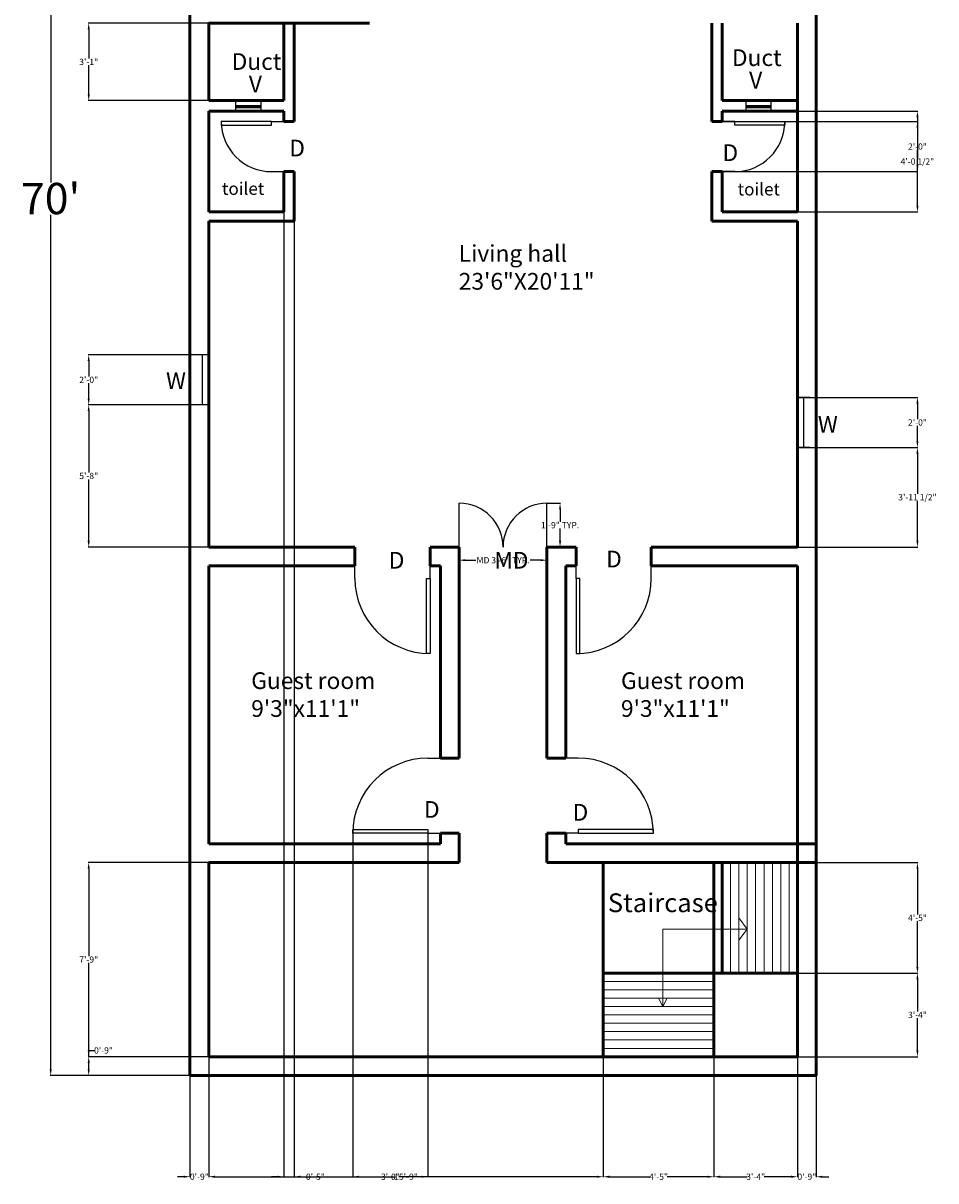
# Model space of a CAD drawing. Units: inches. Extents: x -250 to 2650, y 180 to 1183.
# Tile 7 of 10: x 1594 to 2031, y 180 to 734. Entities that reach past the tile are written whole.
import ezdxf

# ---------------------------------------------------------------- set-up
doc = ezdxf.new("R2010")
doc.units = ezdxf.units.IN
doc.header["$MEASUREMENT"] = 0
for name, color, linetype, lineweight in [('A-ANNO-DIMS', 2, 'Continuous', 18), ('A-ANNO-TEXT', 7, 'Continuous', 18), ('A-AREA-IDEN', 3, 'Continuous', 18), ('A-DOOR', 4, 'Continuous', 25), ('A-FLOR-STRS', 8, 'Continuous', 18), ('A-GLAZ', 3, 'Continuous', 25), ('A-WALL', 7, 'Continuous', 50)]:
    doc.layers.add(name, color=color, linetype=linetype, lineweight=lineweight)
doc.styles.get("Standard").update_dxf_attribs({"font": 'arial.ttf'})
doc.dimstyles.get("Standard").update_dxf_attribs({"dimtxt": 3, "dimasz": 3, "dimexe": 0.18, "dimexo": 0.0625, "dimgap": 0.09, "dimtad": 0, "dimtih": 1, "dimtoh": 1, "dimdec": 0, "dimzin": 0, "dimdsep": 46, "dimlunit": 3, "dimtxsty": 'Standard', "dimcen": 0.09, "dimadec": 0, "dimazin": 0, "dimtfac": 1, "dimtdec": 0, "dimtofl": 0, "dimtmove": 0, "dimatfit": 3, "dimfxl": 1, "dimtolj": 1, "dimtzin": 0, "dimarcsym": 0})

# ---------------------------------------------------------------- blocks, each defined once
blk = doc.blocks.new('*D37')
at = {"layer": 'A-ANNO-DIMS', "color": 0, "lineweight": -2, "transparency": 16777216}
for p, q in [((1673.43, 1070.02), (1606.61, 1070.02)), ((1606.79, 1067.02), (1606.79, 657.77)), ((1606.79, 233.02), (1606.79, 642.28)), ((1673.43, 230.02), (1606.61, 230.02))]:
    blk.add_line(p, q, dxfattribs=at)
at = {"layer": 'A-ANNO-DIMS', "color": 0, "transparency": 16777216}
for points in [[(1606.29, 1067.02), (1607.29, 1067.02), (1606.79, 1070.02)], [(1606.29, 233.02), (1607.29, 233.02), (1606.79, 230.02)]]:
    blk.add_solid(points, dxfattribs=at)
at = {"layer": 'Defpoints', "color": 0, "transparency": 16777216}
for p in [(1673.49, 1070.02), (1606.79, 230.02), (1673.49, 230.02)]:
    blk.add_point(p, dxfattribs=at)
at = {"layer": 'A-ANNO-DIMS', "color": 0, "transparency": 16777216, "insert": (1606.79, 650.02), "char_height": 3, "attachment_point": 5}
blk.add_mtext("\\A1;{\\H5x;70'}", dxfattribs=at)
blk = doc.blocks.new('*U27')
for p, q in [((0, 0), (0, -6)), ((24, 0), (24, -6))]:
    blk.add_line(p, q)
blk.add_lwpolyline([(0, 0), (0, 24), (1.75, 24), (1.75, 0)], close=True)
blk.add_arc((0, 0), 24, 0, 90)
blk = doc.blocks.new('*U28')
for p, q in [((0, 0), (0, 6)), ((24, 0), (24, 6))]:
    blk.add_line(p, q)
blk.add_lwpolyline([(0, 0), (0, -24), (1.75, -24), (1.75, 0)], close=True)
blk.add_arc((0, 0), 24, 270, 0)
blk = doc.blocks.new('*U29')
for p, q in [((0, 5), (0, 0)), ((0, 2.5), (12, 2.5)), ((12, 5), (12, 0))]:
    blk.add_line(p, q)
blk = doc.blocks.new('*U30')
for p, q in [((-36, 0), (-36, -6)), ((0, 0), (0, -6))]:
    blk.add_line(p, q)
blk.add_lwpolyline([(0, 0), (0, 36), (-1.75, 36), (-1.75, 0)], close=True)
blk.add_arc((0, 0), 36, 90, 180)
blk = doc.blocks.new('*U31')
for p, q in [((-36, 0), (-36, 6)), ((0, 0), (0, 6))]:
    blk.add_line(p, q)
blk.add_lwpolyline([(0, 0), (0, -36), (-1.75, -36), (-1.75, 0)], close=True)
blk.add_arc((0, 0), 36, 180, 270)
blk = doc.blocks.new('*U32')
for p, q in [((0, 0), (0, -6)), ((36, 0), (36, -6))]:
    blk.add_line(p, q)
blk.add_lwpolyline([(0, 0), (0, 36), (1.75, 36), (1.75, 0)], close=True)
blk.add_arc((0, 0), 36, 0, 90)
blk = doc.blocks.new('*U33')
for p, q in [((-36, 0), (-36, -6)), ((0, 0), (0, -6))]:
    blk.add_line(p, q)
blk.add_lwpolyline([(0, 0), (0, 36), (-1.75, 36), (-1.75, 0)], close=True)
blk.add_arc((0, 0), 36, 90, 180)
blk = doc.blocks.new('*U23')
for p, q in [((-24, 6), (-24, 0)), ((0, 6), (0, 0)), ((0, 3), (-24, 3))]:
    blk.add_line(p, q)
blk = doc.blocks.new('*U24')
for p, q in [((-24, 6), (-24, 0)), ((0, 6), (0, 0)), ((0, 3), (-24, 3))]:
    blk.add_line(p, q)
blk = doc.blocks.new('DOOR-DOUBLE-MAIN')
for p, q in [((505.08, 483.11), (505.08, 504.11)), ((505.08, 483.11), (505.08, 504.11)), ((547.08, 483.11), (547.08, 504.11))]:
    blk.add_line(p, q)
for centre, start, end in [((505.08, 483.11), 0, 90), ((505.08, 483.11), 0, 90), ((547.08, 483.11), 90, 180)]:
    blk.add_arc(centre, 21, start, end)
blk = doc.blocks.new('*D52')
at = {"layer": 'A-ANNO-DIMS', "color": 0, "lineweight": -2, "transparency": 16777216}
for p, q in [((1802.49, 483.05), (1802.49, 476.63)), ((1844.49, 483.05), (1844.49, 476.63)), ((1805.49, 476.81), (1810.49, 476.81)), ((1841.49, 476.81), (1836.5, 476.81))]:
    blk.add_line(p, q, dxfattribs=at)
at = {"layer": 'A-ANNO-DIMS', "color": 0, "transparency": 16777216}
for points in [[(1805.49, 477.31), (1805.49, 476.31), (1802.49, 476.81)], [(1841.49, 477.31), (1841.49, 476.31), (1844.49, 476.81)]]:
    blk.add_solid(points, dxfattribs=at)
at = {"layer": 'Defpoints', "color": 0, "transparency": 16777216}
for p in [(1802.49, 483.11), (1844.49, 483.11), (1844.49, 476.81)]:
    blk.add_point(p, dxfattribs=at)
at = {"layer": 'A-ANNO-DIMS', "color": 0, "transparency": 16777216, "insert": (1823.49, 476.81), "char_height": 3, "attachment_point": 5}
blk.add_mtext('\\A1;MD 3\'-6" TYP.', dxfattribs=at)
blk = doc.blocks.new('*D53')
at = {"layer": 'A-ANNO-DIMS', "color": 0, "lineweight": -2, "transparency": 16777216}
for p, q in [((1844.55, 504.11), (1850.97, 504.11)), ((1850.79, 501.11), (1850.79, 495.23)), ((1850.79, 486.11), (1850.79, 491.99)), ((1844.55, 483.11), (1850.97, 483.11))]:
    blk.add_line(p, q, dxfattribs=at)
at = {"layer": 'A-ANNO-DIMS', "color": 0, "transparency": 16777216}
for points in [[(1850.29, 501.11), (1851.29, 501.11), (1850.79, 504.11)], [(1850.29, 486.11), (1851.29, 486.11), (1850.79, 483.11)]]:
    blk.add_solid(points, dxfattribs=at)
at = {"layer": 'Defpoints', "color": 0, "transparency": 16777216}
for p in [(1844.49, 504.11), (1850.79, 504.11), (1844.49, 483.11)]:
    blk.add_point(p, dxfattribs=at)
at = {"layer": 'A-ANNO-DIMS', "color": 0, "transparency": 16777216, "insert": (1850.79, 493.61), "char_height": 3, "attachment_point": 5}
blk.add_mtext('\\A1;1\'-9" TYP.', dxfattribs=at)
blk = doc.blocks.new('*D134')
at = {"layer": 'A-ANNO-DIMS', "color": 0, "lineweight": -2, "transparency": 16777216}
for p, q in [((1964.49229, 238.962048), (1964.49229, 181.344548)), ((1973.49229, 229.962048), (1973.49229, 181.344548)), ((1961.49229, 181.524548), (1958.49229, 181.524548)), ((1976.49229, 181.524548), (1979.49229, 181.524548))]:
    blk.add_line(p, q, dxfattribs=at)
at = {"layer": 'A-ANNO-DIMS', "color": 0, "transparency": 16777216}
for points in [[(1961.49229, 182.024548), (1961.49229, 181.024548), (1964.49229, 181.524548)], [(1976.49229, 182.024548), (1976.49229, 181.024548), (1973.49229, 181.524548)]]:
    blk.add_solid(points, dxfattribs=at)
at = {"layer": 'Defpoints', "color": 0, "transparency": 16777216}
for p in [(1964.49229, 239.024548), (1973.49229, 230.024548), (1973.49229, 181.524548)]:
    blk.add_point(p, dxfattribs=at)
at = {"layer": 'A-ANNO-DIMS', "color": 0, "transparency": 16777216, "insert": (1968.99229, 181.524548), "char_height": 3, "attachment_point": 5}
blk.add_mtext('\\A1;0\'-9"', dxfattribs=at)
blk = doc.blocks.new('*D135')
at = {"layer": 'A-ANNO-DIMS', "color": 0, "lineweight": -2, "transparency": 16777216}
for p, q in [((1682.49229, 238.962048), (1682.49229, 181.344548)), ((1673.49229, 229.962048), (1673.49229, 181.344548)), ((1670.49229, 181.524548), (1667.49229, 181.524548)), ((1685.49229, 181.524548), (1688.49229, 181.524548))]:
    blk.add_line(p, q, dxfattribs=at)
at = {"layer": 'A-ANNO-DIMS', "color": 0, "transparency": 16777216}
for points in [[(1670.49229, 182.024548), (1670.49229, 181.024548), (1673.49229, 181.524548)], [(1685.49229, 182.024548), (1685.49229, 181.024548), (1682.49229, 181.524548)]]:
    blk.add_solid(points, dxfattribs=at)
at = {"layer": 'Defpoints', "color": 0, "transparency": 16777216}
for p in [(1682.49229, 239.024548), (1673.49229, 230.024548), (1682.49229, 181.524548)]:
    blk.add_point(p, dxfattribs=at)
at = {"layer": 'A-ANNO-DIMS', "color": 0, "transparency": 16777216, "insert": (1677.99229, 181.524548), "char_height": 3, "attachment_point": 5}
blk.add_mtext('\\A1;0\'-9"', dxfattribs=at)
blk = doc.blocks.new('*D136')
at = {"layer": 'A-ANNO-DIMS', "color": 0, "lineweight": -2, "transparency": 16777216}
for p, q in [((1682.49, 238.96), (1682.49, 181.34)), ((1871.49, 238.96), (1871.49, 181.34)), ((1685.49, 181.52), (1771.89, 181.52)), ((1868.49, 181.52), (1782.09, 181.52))]:
    blk.add_line(p, q, dxfattribs=at)
at = {"layer": 'A-ANNO-DIMS', "color": 0, "transparency": 16777216}
for points in [[(1685.49, 182.02), (1685.49, 181.02), (1682.49, 181.52)], [(1868.49, 182.02), (1868.49, 181.02), (1871.49, 181.52)]]:
    blk.add_solid(points, dxfattribs=at)
at = {"layer": 'Defpoints', "color": 0, "transparency": 16777216}
for p in [(1682.49, 239.02), (1871.49, 239.02), (1871.49, 181.52)]:
    blk.add_point(p, dxfattribs=at)
at = {"layer": 'A-ANNO-DIMS', "color": 0, "transparency": 16777216, "insert": (1776.99, 181.52), "char_height": 3, "attachment_point": 5}
blk.add_mtext('\\A1;15\'-9"', dxfattribs=at)
blk = doc.blocks.new('*D137')
at = {"layer": 'A-ANNO-DIMS', "color": 0, "lineweight": -2, "transparency": 16777216}
for p, q in [((1871.49, 238.96), (1871.49, 181.34)), ((1924.49, 238.96), (1924.49, 181.34)), ((1874.49, 181.52), (1893.85, 181.52)), ((1921.49, 181.52), (1902.13, 181.52))]:
    blk.add_line(p, q, dxfattribs=at)
at = {"layer": 'A-ANNO-DIMS', "color": 0, "transparency": 16777216}
for points in [[(1874.49, 182.02), (1874.49, 181.02), (1871.49, 181.52)], [(1921.49, 182.02), (1921.49, 181.02), (1924.49, 181.52)]]:
    blk.add_solid(points, dxfattribs=at)
at = {"layer": 'Defpoints', "color": 0, "transparency": 16777216}
for p in [(1871.49, 239.02), (1924.49, 239.02), (1924.49, 181.52)]:
    blk.add_point(p, dxfattribs=at)
at = {"layer": 'A-ANNO-DIMS', "color": 0, "transparency": 16777216, "insert": (1897.99, 181.52), "char_height": 3, "attachment_point": 5}
blk.add_mtext('\\A1;4\'-5"', dxfattribs=at)
blk = doc.blocks.new('*D138')
at = {"layer": 'A-ANNO-DIMS', "color": 0, "lineweight": -2, "transparency": 16777216}
for p, q in [((1924.49, 238.96), (1924.49, 181.34)), ((1964.49, 238.96), (1964.49, 181.34)), ((1927.49, 181.52), (1940.42, 181.52)), ((1961.49, 181.52), (1948.57, 181.52))]:
    blk.add_line(p, q, dxfattribs=at)
at = {"layer": 'A-ANNO-DIMS', "color": 0, "transparency": 16777216}
for points in [[(1927.49, 182.02), (1927.49, 181.02), (1924.49, 181.52)], [(1961.49, 182.02), (1961.49, 181.02), (1964.49, 181.52)]]:
    blk.add_solid(points, dxfattribs=at)
at = {"layer": 'Defpoints', "color": 0, "transparency": 16777216}
for p in [(1924.49, 239.02), (1964.49, 239.02), (1964.49, 181.52)]:
    blk.add_point(p, dxfattribs=at)
at = {"layer": 'A-ANNO-DIMS', "color": 0, "transparency": 16777216, "insert": (1944.49, 181.52), "char_height": 3, "attachment_point": 5}
blk.add_mtext('\\A1;3\'-4"', dxfattribs=at)
blk = doc.blocks.new('*D139')
at = {"layer": 'A-ANNO-DIMS', "color": 0, "lineweight": -2, "transparency": 16777216}
for p, q in [((1964.55, 279.02), (2022.17, 279.02)), ((2021.99, 276.02), (2021.99, 260.65)), ((2021.99, 242.02), (2021.99, 257.4)), ((1964.55, 239.02), (2022.17, 239.02))]:
    blk.add_line(p, q, dxfattribs=at)
at = {"layer": 'A-ANNO-DIMS', "color": 0, "transparency": 16777216}
for points in [[(2021.49, 276.02), (2022.49, 276.02), (2021.99, 279.02)], [(2021.49, 242.02), (2022.49, 242.02), (2021.99, 239.02)]]:
    blk.add_solid(points, dxfattribs=at)
at = {"layer": 'Defpoints', "color": 0, "transparency": 16777216}
for p in [(1964.49, 279.02), (2021.99, 279.02), (1964.49, 239.02)]:
    blk.add_point(p, dxfattribs=at)
at = {"layer": 'A-ANNO-DIMS', "color": 0, "transparency": 16777216, "insert": (2021.99, 259.02), "char_height": 3, "attachment_point": 5}
blk.add_mtext('\\A1;3\'-4"', dxfattribs=at)
blk = doc.blocks.new('*D140')
at = {"layer": 'A-ANNO-DIMS', "color": 0, "lineweight": -2, "transparency": 16777216}
for p, q in [((1960.55, 332.02), (2022.17, 332.02)), ((2021.99, 329.02), (2021.99, 307.14)), ((2021.99, 282.02), (2021.99, 303.91)), ((1964.55, 279.02), (2022.17, 279.02))]:
    blk.add_line(p, q, dxfattribs=at)
at = {"layer": 'A-ANNO-DIMS', "color": 0, "transparency": 16777216}
for points in [[(2021.49, 329.02), (2022.49, 329.02), (2021.99, 332.02)], [(2021.49, 282.02), (2022.49, 282.02), (2021.99, 279.02)]]:
    blk.add_solid(points, dxfattribs=at)
at = {"layer": 'Defpoints', "color": 0, "transparency": 16777216}
for p in [(1960.49, 332.02), (2021.99, 332.02), (1964.49, 279.02)]:
    blk.add_point(p, dxfattribs=at)
at = {"layer": 'A-ANNO-DIMS', "color": 0, "transparency": 16777216, "insert": (2021.99, 305.52), "char_height": 3, "attachment_point": 5}
blk.add_mtext('\\A1;4\'-5"', dxfattribs=at)
blk = doc.blocks.new('*D141')
at = {"layer": 'A-ANNO-DIMS', "color": 0, "lineweight": -2, "transparency": 16777216}
for p, q in [((1682.43, 239.02), (1624.81, 239.02)), ((1624.99, 239.02), (1624.99, 242.02)), ((1624.99, 242.02), (1627.99, 242.02)), ((1624.99, 233.02), (1624.99, 236.02)), ((1673.43, 230.02), (1624.81, 230.02))]:
    blk.add_line(p, q, dxfattribs=at)
at = {"layer": 'A-ANNO-DIMS', "color": 0, "transparency": 16777216}
for points in [[(1624.49, 236.02), (1625.49, 236.02), (1624.99, 239.02)], [(1624.49, 233.02), (1625.49, 233.02), (1624.99, 230.02)]]:
    blk.add_solid(points, dxfattribs=at)
at = {"layer": 'Defpoints', "color": 0, "transparency": 16777216}
for p in [(1624.99, 239.02), (1682.49, 239.02), (1673.49, 230.02)]:
    blk.add_point(p, dxfattribs=at)
at = {"layer": 'A-ANNO-DIMS', "color": 0, "transparency": 16777216, "insert": (1632.07, 242.02), "char_height": 3, "attachment_point": 5}
blk.add_mtext('\\A1;0\'-9"', dxfattribs=at)
blk = doc.blocks.new('*D142')
at = {"layer": 'A-ANNO-DIMS', "color": 0, "lineweight": -2, "transparency": 16777216}
for p, q in [((1682.43, 332.02), (1624.81, 332.02)), ((1624.99, 329.02), (1624.99, 287.15)), ((1624.99, 242.02), (1624.99, 283.9)), ((1682.43, 239.02), (1624.81, 239.02))]:
    blk.add_line(p, q, dxfattribs=at)
at = {"layer": 'A-ANNO-DIMS', "color": 0, "transparency": 16777216}
for points in [[(1624.49, 329.02), (1625.49, 329.02), (1624.99, 332.02)], [(1624.49, 242.02), (1625.49, 242.02), (1624.99, 239.02)]]:
    blk.add_solid(points, dxfattribs=at)
at = {"layer": 'Defpoints', "color": 0, "transparency": 16777216}
for p in [(1624.99, 332.02), (1682.49, 332.02), (1682.49, 239.02)]:
    blk.add_point(p, dxfattribs=at)
at = {"layer": 'A-ANNO-DIMS', "color": 0, "transparency": 16777216, "insert": (1624.99, 285.52), "char_height": 3, "attachment_point": 5}
blk.add_mtext('\\A1;7\'-9"', dxfattribs=at)
blk = doc.blocks.new('*D144')
at = {"layer": 'A-ANNO-DIMS', "color": 0, "lineweight": -2, "transparency": 16777216}
for p, q in [((1718.49, 643.56), (1718.49, 181.34)), ((1723.49, 639.05), (1723.49, 181.34)), ((1715.49, 181.52), (1712.49, 181.52)), ((1726.49, 181.52), (1729.49, 181.52))]:
    blk.add_line(p, q, dxfattribs=at)
at = {"layer": 'A-ANNO-DIMS', "color": 0, "transparency": 16777216}
for points in [[(1715.49, 182.02), (1715.49, 181.02), (1718.49, 181.52)], [(1726.49, 182.02), (1726.49, 181.02), (1723.49, 181.52)]]:
    blk.add_solid(points, dxfattribs=at)
at = {"layer": 'Defpoints', "color": 0, "transparency": 16777216}
for p in [(1718.49, 643.62), (1723.49, 639.11), (1723.49, 181.52)]:
    blk.add_point(p, dxfattribs=at)
at = {"layer": 'A-ANNO-DIMS', "color": 0, "transparency": 16777216, "insert": (1733.57, 181.52), "char_height": 3, "attachment_point": 5}
blk.add_mtext('\\A1;0\'-5"', dxfattribs=at)
blk = doc.blocks.new('*D145')
at = {"layer": 'A-ANNO-DIMS', "color": 0, "lineweight": -2, "transparency": 16777216}
for p, q in [((1682.43, 734.02), (1624.81, 734.02)), ((1624.99, 731.02), (1624.99, 717.09)), ((1624.99, 699.91), (1624.99, 713.84)), ((1682.43, 696.91), (1624.81, 696.91))]:
    blk.add_line(p, q, dxfattribs=at)
at = {"layer": 'A-ANNO-DIMS', "color": 0, "transparency": 16777216}
for points in [[(1624.49, 731.02), (1625.49, 731.02), (1624.99, 734.02)], [(1624.49, 699.91), (1625.49, 699.91), (1624.99, 696.91)]]:
    blk.add_solid(points, dxfattribs=at)
at = {"layer": 'Defpoints', "color": 0, "transparency": 16777216}
for p in [(1624.99, 734.02), (1682.49, 734.02), (1682.49, 696.91)]:
    blk.add_point(p, dxfattribs=at)
at = {"layer": 'A-ANNO-DIMS', "color": 0, "transparency": 16777216, "insert": (1624.99, 715.47), "char_height": 3, "attachment_point": 5}
blk.add_mtext('\\A1;3\'-1"', dxfattribs=at)
blk = doc.blocks.new('*D146')
at = {"layer": 'A-ANNO-DIMS', "color": 0, "lineweight": -2, "transparency": 16777216}
for p, q in [((1964.55, 691.91), (2022.17, 691.91)), ((2021.99, 688.91), (2021.99, 669.41)), ((2021.99, 646.62), (2021.99, 666.12)), ((1964.55, 643.62), (2022.17, 643.62))]:
    blk.add_line(p, q, dxfattribs=at)
at = {"layer": 'A-ANNO-DIMS', "color": 0, "transparency": 16777216}
for points in [[(2021.49, 688.91), (2022.49, 688.91), (2021.99, 691.91)], [(2021.49, 646.62), (2022.49, 646.62), (2021.99, 643.62)]]:
    blk.add_solid(points, dxfattribs=at)
at = {"layer": 'Defpoints', "color": 0, "transparency": 16777216}
for p in [(1964.49, 691.91), (2021.99, 691.91), (1964.49, 643.62)]:
    blk.add_point(p, dxfattribs=at)
at = {"layer": 'A-ANNO-DIMS', "color": 0, "transparency": 16777216, "insert": (2021.99, 667.77), "char_height": 3, "attachment_point": 5}
blk.add_mtext('\\A1;4\'-0 1/2"', dxfattribs=at)
blk = doc.blocks.new('*D147')
at = {"layer": 'A-ANNO-DIMS', "color": 0, "lineweight": -2, "transparency": 16777216}
for p, q in [((1964.55, 530.79), (2022.17, 530.79)), ((2021.99, 527.79), (2021.99, 508.59)), ((2021.99, 486.11), (2021.99, 505.31)), ((1964.55, 483.11), (2022.17, 483.11))]:
    blk.add_line(p, q, dxfattribs=at)
at = {"layer": 'A-ANNO-DIMS', "color": 0, "transparency": 16777216}
for points in [[(2021.49, 527.79), (2022.49, 527.79), (2021.99, 530.79)], [(2021.49, 486.11), (2022.49, 486.11), (2021.99, 483.11)]]:
    blk.add_solid(points, dxfattribs=at)
at = {"layer": 'Defpoints', "color": 0, "transparency": 16777216}
for p in [(1964.49, 530.79), (2021.99, 530.79), (1964.49, 483.11)]:
    blk.add_point(p, dxfattribs=at)
at = {"layer": 'A-ANNO-DIMS', "color": 0, "transparency": 16777216, "insert": (2021.99, 506.95), "char_height": 3, "attachment_point": 5}
blk.add_mtext('\\A1;3\'-11 1/2"', dxfattribs=at)
blk = doc.blocks.new('*D148')
at = {"layer": 'A-ANNO-DIMS', "color": 0, "lineweight": -2, "transparency": 16777216}
for p, q in [((1964.55, 554.79), (2022.17, 554.79)), ((2021.99, 551.79), (2021.99, 544.41)), ((2021.99, 533.79), (2021.99, 541.16)), ((1964.55, 530.79), (2022.17, 530.79))]:
    blk.add_line(p, q, dxfattribs=at)
at = {"layer": 'A-ANNO-DIMS', "color": 0, "transparency": 16777216}
for points in [[(2021.49, 551.79), (2022.49, 551.79), (2021.99, 554.79)], [(2021.49, 533.79), (2022.49, 533.79), (2021.99, 530.79)]]:
    blk.add_solid(points, dxfattribs=at)
at = {"layer": 'Defpoints', "color": 0, "transparency": 16777216}
for p in [(1964.49, 554.79), (2021.99, 554.79), (1964.49, 530.79)]:
    blk.add_point(p, dxfattribs=at)
at = {"layer": 'A-ANNO-DIMS', "color": 0, "transparency": 16777216, "insert": (2021.99, 542.79), "char_height": 3, "attachment_point": 5}
blk.add_mtext('\\A1;2\'-0"', dxfattribs=at)
blk = doc.blocks.new('*D149')
at = {"layer": 'A-ANNO-DIMS', "color": 0, "lineweight": -2, "transparency": 16777216}
for p, q in [((1682.43, 551.2), (1624.81, 551.2)), ((1624.99, 548.2), (1624.99, 518.78)), ((1624.99, 486.11), (1624.99, 515.53)), ((1682.43, 483.11), (1624.81, 483.11))]:
    blk.add_line(p, q, dxfattribs=at)
at = {"layer": 'A-ANNO-DIMS', "color": 0, "transparency": 16777216}
for points in [[(1624.49, 548.2), (1625.49, 548.2), (1624.99, 551.2)], [(1624.49, 486.11), (1625.49, 486.11), (1624.99, 483.11)]]:
    blk.add_solid(points, dxfattribs=at)
at = {"layer": 'Defpoints', "color": 0, "transparency": 16777216}
for p in [(1624.99, 551.2), (1682.49, 551.2), (1682.49, 483.11)]:
    blk.add_point(p, dxfattribs=at)
at = {"layer": 'A-ANNO-DIMS', "color": 0, "transparency": 16777216, "insert": (1624.99, 517.16), "char_height": 3, "attachment_point": 5}
blk.add_mtext('\\A1;5\'-8"', dxfattribs=at)
blk = doc.blocks.new('*D150')
at = {"layer": 'A-ANNO-DIMS', "color": 0, "lineweight": -2, "transparency": 16777216}
for p, q in [((1682.43, 575.2), (1624.81, 575.2)), ((1624.99, 572.2), (1624.99, 564.82)), ((1624.99, 554.2), (1624.99, 561.58)), ((1682.43, 551.2), (1624.81, 551.2))]:
    blk.add_line(p, q, dxfattribs=at)
at = {"layer": 'A-ANNO-DIMS', "color": 0, "transparency": 16777216}
for points in [[(1624.49, 572.2), (1625.49, 572.2), (1624.99, 575.2)], [(1624.49, 554.2), (1625.49, 554.2), (1624.99, 551.2)]]:
    blk.add_solid(points, dxfattribs=at)
at = {"layer": 'Defpoints', "color": 0, "transparency": 16777216}
for p in [(1624.99, 575.2), (1682.49, 575.2), (1682.49, 551.2)]:
    blk.add_point(p, dxfattribs=at)
at = {"layer": 'A-ANNO-DIMS', "color": 0, "transparency": 16777216, "insert": (1624.99, 563.2), "char_height": 3, "attachment_point": 5}
blk.add_mtext('\\A1;2\'-0"', dxfattribs=at)
blk = doc.blocks.new('*D151')
at = {"layer": 'A-ANNO-DIMS', "color": 0, "lineweight": -2, "transparency": 16777216}
for p, q in [((1751.49, 345.96), (1751.49, 181.34)), ((1787.49, 345.96), (1787.49, 181.34)), ((1754.49, 181.52), (1765.42, 181.52)), ((1784.49, 181.52), (1773.57, 181.52))]:
    blk.add_line(p, q, dxfattribs=at)
at = {"layer": 'A-ANNO-DIMS', "color": 0, "transparency": 16777216}
for points in [[(1754.49, 182.02), (1754.49, 181.02), (1751.49, 181.52)], [(1784.49, 182.02), (1784.49, 181.02), (1787.49, 181.52)]]:
    blk.add_solid(points, dxfattribs=at)
at = {"layer": 'Defpoints', "color": 0, "transparency": 16777216}
for p in [(1751.49, 346.02), (1787.49, 346.02), (1787.49, 181.52)]:
    blk.add_point(p, dxfattribs=at)
at = {"layer": 'A-ANNO-DIMS', "color": 0, "transparency": 16777216, "insert": (1769.49, 181.52), "char_height": 3, "attachment_point": 5}
blk.add_mtext('\\A1;3\'-0"', dxfattribs=at)
blk = doc.blocks.new('*D152')
at = {"layer": 'A-ANNO-DIMS', "color": 0, "lineweight": -2, "transparency": 16777216}
for p, q in [((1923.55, 686.91), (2022.17, 686.91)), ((2021.99, 683.91), (2021.99, 676.53)), ((2021.99, 665.91), (2021.99, 673.29)), ((1923.55, 662.91), (2022.17, 662.91))]:
    blk.add_line(p, q, dxfattribs=at)
at = {"layer": 'A-ANNO-DIMS', "color": 0, "transparency": 16777216}
for points in [[(2021.49, 683.91), (2022.49, 683.91), (2021.99, 686.91)], [(2021.49, 665.91), (2022.49, 665.91), (2021.99, 662.91)]]:
    blk.add_solid(points, dxfattribs=at)
at = {"layer": 'Defpoints', "color": 0, "transparency": 16777216}
for p in [(1923.49, 686.91), (2021.99, 686.91), (1923.49, 662.91)]:
    blk.add_point(p, dxfattribs=at)
at = {"layer": 'A-ANNO-DIMS', "color": 0, "transparency": 16777216, "insert": (2021.99, 674.91), "char_height": 3, "attachment_point": 5}
blk.add_mtext('\\A1;2\'-0"', dxfattribs=at)

msp = doc.modelspace()

# ---------------------------------------------------------------- linework, layer by layer
at = {"layer": 'A-FLOR-STRS'}
for p, q in [((1932.49, 279.02), (1932.49, 332.02)), ((1936.49, 279.02), (1936.49, 332.02)), ((1940.49, 279.02), (1940.49, 332.02)), ((1944.49, 279.02), (1944.49, 332.02)), ((1948.49, 279.02), (1948.49, 332.02)), ((1952.49, 279.02), (1952.49, 332.02)), ((1956.49, 279.02), (1956.49, 332.02)), ((1960.49, 279.02), (1960.49, 332.02)), ((1940.49, 300.14), (1936.49, 305.52)), ((1900, 300.14), (1900, 263.02)), ((1900, 300.14), (1940.49, 300.14)), ((1940.49, 300.14), (1936.49, 294.75)), ((1871.49, 275.02), (1924.49, 275.02)), ((1871.49, 271.02), (1924.49, 271.02)), ((1871.49, 267.02), (1924.49, 267.02)), ((1900, 263.02), (1897.99, 267.02)), ((1900, 263.02), (1902.02, 267.02)), ((1871.49, 263.02), (1924.49, 263.02)), ((1871.49, 259.02), (1924.49, 259.02)), ((1871.49, 255.02), (1924.49, 255.02)), ((1871.49, 251.02), (1924.49, 251.02)), ((1871.49, 247.02), (1924.49, 247.02)), ((1871.49, 243.02), (1924.49, 243.02))]:
    msp.add_line(p, q, dxfattribs=at)
at = {"layer": 'A-WALL'}
for p, q in [((1673.49, 1070.02), (1673.49, 230.02)), ((1973.49, 230.02), (1973.49, 1070.02)), ((1759.49, 734.02), (1682.49, 734.02)), ((1682.49, 734.02), (1682.49, 696.91)), ((1718.49, 696.91), (1718.49, 734.02)), ((1723.49, 686.91), (1723.49, 734.02)), ((1923.49, 686.91), (1923.49, 734.02)), ((1923.49, 686.91), (1923.49, 734.02)), ((1928.49, 696.91), (1928.49, 734.02)), ((1964.49, 643.62), (1964.49, 734.02)), ((1964.49, 696.91), (1964.49, 734.02)), ((1964.49, 716.02), (1964.49, 734.02)), ((1718.49, 696.91), (1682.49, 696.91)), ((1707.55, 693.93), (1695.55, 693.93)), ((1964.49, 696.91), (1928.49, 696.91)), ((1951.93, 693.93), (1939.93, 693.93)), ((1682.49, 691.91), (1682.49, 643.62)), ((1718.49, 691.91), (1682.49, 691.91)), ((1718.49, 691.91), (1718.49, 686.91)), ((1928.49, 686.91), (1928.49, 691.91)), ((1964.49, 691.91), (1928.49, 691.91)), ((1964.49, 643.62), (1964.49, 691.91)), ((1718.49, 686.91), (1723.49, 686.91)), ((1928.49, 686.91), (1923.49, 686.91)), ((1718.49, 662.91), (1718.49, 643.62)), ((1718.49, 662.91), (1723.49, 662.91)), ((1723.49, 639.11), (1723.49, 662.91)), ((1723.49, 662.91), (1723.49, 639.11)), ((1923.49, 639.11), (1923.49, 662.91)), ((1923.49, 643.62), (1923.49, 662.91)), ((1928.49, 662.91), (1923.49, 662.91)), ((1928.49, 643.62), (1928.49, 662.91)), ((1718.49, 643.62), (1682.49, 643.62)), ((1723.49, 643.62), (1723.49, 643.62)), ((1964.49, 643.62), (1928.49, 643.62)), ((1682.49, 639.11), (1682.49, 483.11)), ((1723.49, 639.11), (1682.49, 639.11)), ((1964.49, 639.11), (1923.49, 639.11)), ((1964.49, 483.11), (1964.49, 639.11)), ((1964.49, 587.02), (1964.49, 639.11)), ((1752.49, 483.11), (1682.49, 483.11)), ((1752.49, 474.11), (1752.49, 483.11)), ((1802.49, 483.11), (1788.49, 483.11)), ((1788.49, 474.11), (1788.49, 483.11)), ((1802.49, 483.11), (1802.49, 382.02)), ((1844.49, 382.02), (1844.49, 483.11)), ((1858.49, 483.11), (1844.49, 483.11)), ((1858.49, 474.11), (1858.49, 483.11)), ((1964.49, 483.11), (1894.49, 483.11)), ((1894.49, 474.11), (1894.49, 483.11)), ((1682.49, 474.11), (1682.49, 341.02)), ((1752.49, 474.11), (1682.49, 474.11)), ((1793.49, 474.11), (1788.49, 474.11)), ((1793.49, 474.11), (1793.49, 382.02)), ((1853.49, 382.02), (1853.49, 474.11)), ((1858.49, 474.11), (1853.49, 474.11)), ((1964.49, 474.11), (1894.49, 474.11)), ((1964.49, 239.02), (1964.49, 474.11)), ((1793.49, 382.02), (1802.49, 382.02)), ((1844.49, 382.02), (1853.49, 382.02)), ((1793.49, 346.02), (1793.49, 341.02)), ((1793.49, 346.02), (1802.49, 346.02)), ((1802.49, 346.02), (1802.49, 332.02)), ((1844.49, 332.02), (1844.49, 346.02)), ((1853.49, 346.02), (1844.49, 346.02)), ((1853.49, 341.02), (1853.49, 346.02)), ((1682.49, 341.02), (1793.49, 341.02)), ((1853.49, 341.02), (1973.49, 341.02)), ((1682.49, 332.02), (1802.49, 332.02)), ((1682.49, 332.02), (1682.49, 239.02)), ((1844.49, 332.02), (1973.49, 332.02)), ((1871.49, 239.02), (1871.49, 332.02)), ((1924.49, 239.02), (1924.49, 332.02)), ((1928.49, 279.02), (1928.49, 332.02)), ((1871.49, 279.02), (1964.49, 279.02)), ((1682.49, 239.02), (1707.24, 239.02)), ((1682.49, 239.02), (1964.49, 239.02)), ((1673.49, 230.02), (1706.49, 230.02)), ((1673.49, 230.02), (1973.49, 230.02))]:
    msp.add_line(p, q, dxfattribs=at)

# ---------------------------------------------------------------- block references
at = {"layer": 'A-DOOR'}
for name, p, rotation in [('*U28', (1712.49, 686.91), 270), ('*U27', (1934.49, 686.91), 270), ('*U32', (1788.49, 468.11), 180), ('*U33', (1858.49, 468.11), 180), ('*U31', (1787.49, 346.02), 270), ('*U30', (1859.49, 346.02), 270)]:
    msp.add_blockref(name, p, dxfattribs=dict(at, rotation=rotation))
msp.add_blockref('DOOR-DOUBLE-MAIN', (1297.41, 0), dxfattribs=at)
at = {"layer": 'A-GLAZ'}
for name, p, rotation in [('*U29', (1707.55, 696.91), 180), ('*U29', (1951.93, 696.91), 180), ('*U23', (1676.49, 551.2), 270), ('*U24', (1964.49, 530.79), 270)]:
    msp.add_blockref(name, p, dxfattribs=dict(at, rotation=rotation))

# ---------------------------------------------------------------- texts
at = {"layer": 'A-ANNO-TEXT', "char_height": 8, "attachment_point": 1}
for s, insert in [('V', (1941.36, 710.71)), ('V', (1701.71, 708.86)), ('D', (1721.07, 678.19)), ('D', (1928.58, 675.98)), ('W', (1662.01, 566.85)), ('W', (1974.27, 545.9)), ('D', (1768.73, 480.78)), ('MD', (1819.3, 480.78)), ('D', (1872.85, 481.35)), ('D', (1785.6, 361.42)), ('D', (1856.8, 360.07))]:
    msp.add_mtext_dynamic_manual_height_columns(s, width=10.3916, gutter_width=1, heights=[0], dxfattribs=dict(at, insert=insert))
at = {"layer": 'A-AREA-IDEN', "attachment_point": 1}
for s, width, heights, insert, char_height in [('{\\H2.66667x;Duct} ', 7.71, [3.05], (1933.11, 721.49), 3), ('{\\H2.66667x;Duct} ', 7.71, [3.05], (1693.46, 719.65), 3), ('toilet', 19.3499, [0], (1688.84, 657.78), 6), ('toilet', 19.3499, [0], (1935.88, 657.5), 6), ('Living hall  \\P23\'6"X20\'11"', 123.5412, [0], (1802.26, 627.72), 8), ('Guest room 9\'3"x11\'1"', 88.0689, [0], (1702.84, 423.12), 8), ('Guest room 9\'3"x11\'1"', 88.0689, [0], (1879.97, 423.12), 8), ('Staircase  ', 87.4783, [0], (1873.67, 317.24), 9)]:
    msp.add_mtext_dynamic_manual_height_columns(s, width=width, gutter_width=1, heights=heights, dxfattribs=dict(at, insert=insert, char_height=char_height))

# ---------------------------------------------------------------- dimensions: what is measured, and where the dimension line sits
at = {"layer": 'A-ANNO-DIMS'}
for base, p1, p2, text, override, picture, middle in [((1606.79, 230.02), (1673.49, 1070.02), (1673.49, 230.02), '{\\H5x;<>}', {"dimclrd": 0, "dimclre": 0, "dimclrt": 0}, '*D37', (1606.79, 650.02)), ((1850.79, 504.11), (1844.49, 483.11), (1844.49, 504.11), '<> TYP.', {"dimdec": 1, "dimrnd": 0, "dimzin": 1, "dimlunit": 4, "dimfrac": 2}, '*D53', (1850.79, 493.61))]:
    dim = msp.add_linear_dim(base=base, p1=p1, p2=p2, angle=90, text=text, dimstyle='Standard', override=override, dxfattribs=at)
    dim.commit()
    dim.dimension.update_dxf_attribs({"geometry": picture, "text_midpoint": middle})
for base, p1, p2, picture, middle in [((1624.99, 734.02), (1682.49, 696.91), (1682.49, 734.02), '*D145', (1624.99, 715.47)), ((2021.99, 691.91), (1964.49, 643.62), (1964.49, 691.91), '*D146', (2021.99, 667.77)), ((2021.99, 686.91), (1923.49, 662.91), (1923.49, 686.91), '*D152', (2021.99, 674.91)), ((1624.99, 575.2), (1682.49, 551.2), (1682.49, 575.2), '*D150', (1624.99, 563.2)), ((2021.99, 554.79), (1964.49, 530.79), (1964.49, 554.79), '*D148', (2021.99, 542.79)), ((1624.99, 551.2), (1682.49, 483.11), (1682.49, 551.2), '*D149', (1624.99, 517.16)), ((2021.99, 530.79), (1964.49, 483.11), (1964.49, 530.79), '*D147', (2021.99, 506.95)), ((1624.99, 332.02), (1682.49, 239.02), (1682.49, 332.02), '*D142', (1624.99, 285.52)), ((2021.99, 332.02), (1964.49, 279.02), (1960.49, 332.02), '*D140', (2021.99, 305.52)), ((2021.99, 279.02), (1964.49, 239.02), (1964.49, 279.02), '*D139', (2021.99, 259.02)), ((1624.99, 239.02), (1673.49, 230.02), (1682.49, 239.02), '*D141', (1632.07, 242.02))]:
    dim = msp.add_linear_dim(base=base, p1=p1, p2=p2, angle=90, dimstyle='Standard', override={"dimdec": 1, "dimlfac": 1, "dimrnd": 0, "dimzin": 1, "dimdsep": 46, "dimlunit": 4, "dimfrac": 2}, dxfattribs=at)
    dim.commit()
    dim.dimension.update_dxf_attribs({"geometry": picture, "text_midpoint": middle})
for base, p1, p2, picture, middle in [((1723.49, 181.52), (1718.49, 643.62), (1723.49, 639.11), '*D144', (1733.57, 181.52)), ((1787.49, 181.52), (1751.49, 346.02), (1787.49, 346.02), '*D151', (1769.49, 181.52)), ((1682.49, 181.52), (1673.49, 230.02), (1682.49, 239.02), '*D135', (1677.99, 181.52)), ((1871.49, 181.52), (1682.49, 239.02), (1871.49, 239.02), '*D136', (1776.99, 181.52)), ((1924.49, 181.52), (1871.49, 239.02), (1924.49, 239.02), '*D137', (1897.99, 181.52)), ((1964.49, 181.52), (1924.49, 239.02), (1964.49, 239.02), '*D138', (1944.49, 181.52)), ((1973.49, 181.52), (1964.49, 239.02), (1973.49, 230.02), '*D134', (1968.99, 181.52))]:
    dim = msp.add_linear_dim(base=base, p1=p1, p2=p2, dimstyle='Standard', override={"dimdec": 1, "dimlfac": 1, "dimrnd": 0, "dimzin": 1, "dimdsep": 46, "dimlunit": 4, "dimfrac": 2}, dxfattribs=at)
    dim.commit()
    dim.dimension.update_dxf_attribs({"geometry": picture, "text_midpoint": middle})
dim = msp.add_linear_dim(base=(1844.49, 476.81), p1=(1802.49, 483.11), p2=(1844.49, 483.11), text='MD <> TYP.', dimstyle='Standard', override={"dimdec": 1, "dimrnd": 0, "dimzin": 1, "dimlunit": 4, "dimfrac": 2}, dxfattribs=at)
dim.commit()
dim.dimension.update_dxf_attribs({"geometry": '*D52', "text_midpoint": (1823.49, 476.81)})

doc.saveas('drawing.dxf')
